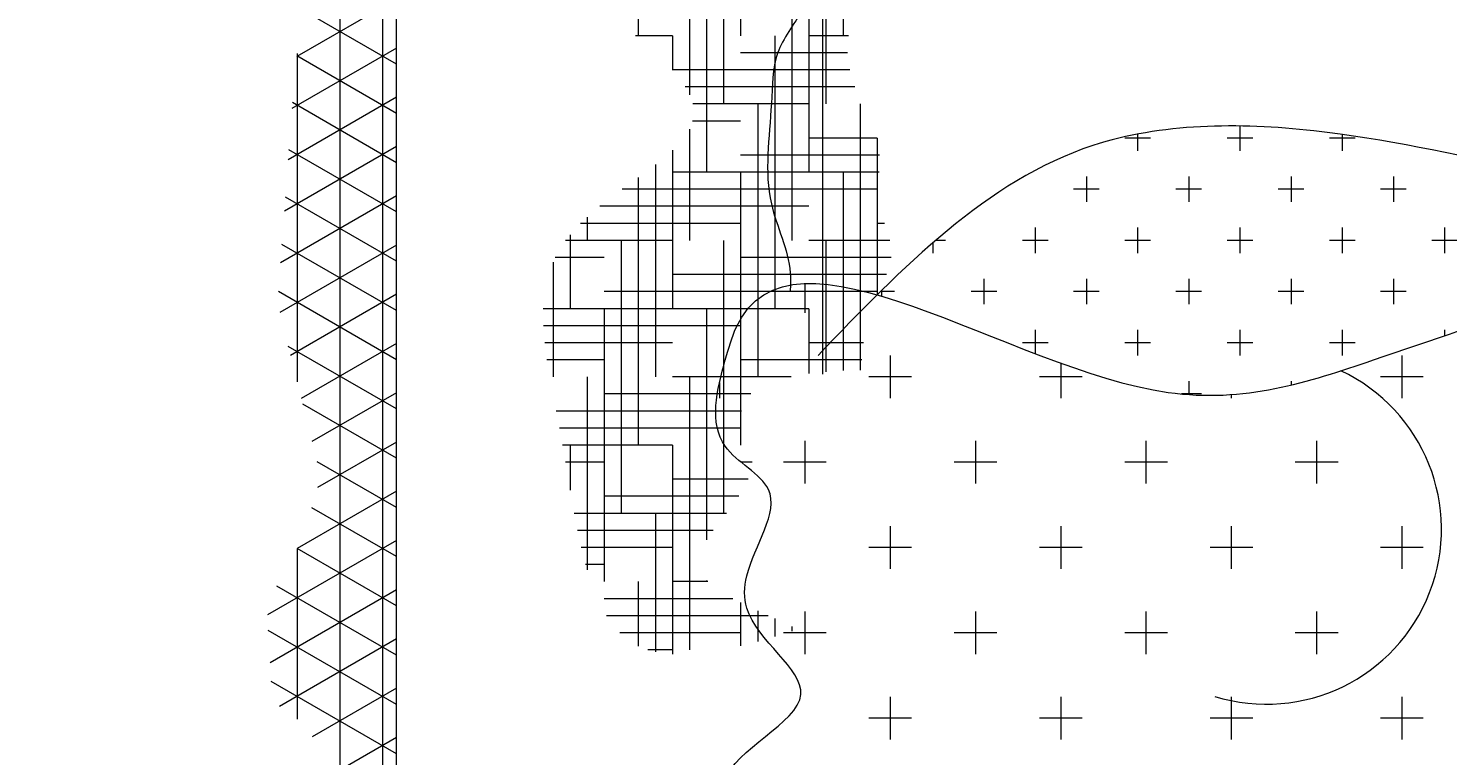
# Model space of a CAD drawing. Units: inches. Extents: x 3731 to 4318, y 1310 to 2388.
# Tile 43 of 57: x 4124 to 4167, y 1977 to 1999. Entities that reach past the tile are written whole.
import ezdxf

# ---------------------------------------------------------------- set-up
doc = ezdxf.new("R2010")
doc.units = ezdxf.units.IN
doc.layers.add('A-ANNO-DIMS', color=2, linetype='Continuous', lineweight=18)
doc.layers.add('A-FURN', color=8, linetype='Continuous', lineweight=13)
doc.styles.get("Standard").update_dxf_attribs({"font": 'arial.ttf'})
doc.dimstyles.get("Standard").update_dxf_attribs({"dimtxt": 0.18, "dimasz": 0.18, "dimexe": 0.18, "dimexo": 0.0625, "dimgap": 0.09, "dimtad": 0, "dimtih": 1, "dimtoh": 1, "dimdec": 4, "dimzin": 0, "dimdsep": 46, "dimtxsty": 'Standard', "dimcen": 0.09, "dimadec": 0, "dimazin": 0, "dimtfac": 1, "dimtdec": 4, "dimtofl": 0, "dimtmove": 0, "dimatfit": 3, "dimfxl": 1, "dimtolj": 1, "dimtzin": 0, "dimarcsym": 0})

# ---------------------------------------------------------------- blocks, each defined once
blk = doc.blocks.new('A$C200C7901')
for p, q in [((2.3121, 1.6596), (2.3121, 0.0201)), ((2, 0.2957), (2, 1.2957)), ((2.0224, 0.9977), (2.0224, 1.1977)), ((2.0224, 0.9977), (2.0224, 1.1977))]:
    blk.add_line(p, q)
at = {"linetype": 'ByBlock'}
for p, q in [((2.3224, 0.0468), (2.3224, 1.6627)), ((2.3224, 0.0468), (2.3224, 1.6627)), ((2.3537, 0.0056), (2.3537, 1.634)), ((2.3537, 0.0056), (2.3537, 1.634)), ((2.3121, 1.5619), (2.3654, 1.5926)), ((2.3121, 1.5619), (2.3654, 1.5926)), ((2.3121, 1.5738), (2.404, 1.5208)), ((2.3121, 1.5738), (2.404, 1.5208)), ((1.5754, 1.532), (1.5754, 1.5633)), ((1.5754, 1.532), (1.5754, 1.5633)), ((1.7004, 1.532), (1.7004, 1.5633)), ((1.7004, 1.532), (1.7004, 1.5633)), ((1.8254, 1.532), (1.8254, 1.5633)), ((1.8254, 1.532), (1.8254, 1.5633)), ((1.9504, 1.532), (1.9504, 1.5633)), ((1.9504, 1.532), (1.9504, 1.5633)), ((2.3121, 1.5258), (2.3739, 1.5615)), ((2.3121, 1.5258), (2.3739, 1.5615)), ((1.5597, 1.5477), (1.591, 1.5477)), ((1.5597, 1.5477), (1.591, 1.5477)), ((1.6847, 1.5477), (1.716, 1.5477)), ((1.6847, 1.5477), (1.716, 1.5477)), ((1.8097, 1.5477), (1.841, 1.5477)), ((1.8097, 1.5477), (1.841, 1.5477)), ((1.9347, 1.5477), (1.966, 1.5477)), ((1.9347, 1.5477), (1.966, 1.5477)), ((2.3121, 1.4897), (2.3979, 1.5393)), ((2.3121, 1.4897), (2.3979, 1.5393)), ((2.3849, 1.4236), (2.3849, 1.5486)), ((2.3849, 1.4236), (2.3849, 1.5486)), ((2.3121, 1.5377), (2.406, 1.4835)), ((2.3121, 1.5377), (2.406, 1.4835)), ((1.6379, 1.4695), (1.6379, 1.5008)), ((1.6379, 1.4695), (1.6379, 1.5008)), ((1.7629, 1.4695), (1.7629, 1.5008)), ((1.7629, 1.4695), (1.7629, 1.5008)), ((1.8879, 1.4695), (1.8879, 1.5008)), ((1.8879, 1.4695), (1.8879, 1.5008)), ((2.0129, 1.4695), (2.0129, 1.5008)), ((2.0129, 1.4695), (2.0129, 1.5008)), ((2.0974, 1.2977), (2.0974, 1.4977)), ((2.0974, 1.2977), (2.0974, 1.4977)), ((2.1099, 1.3477), (2.1099, 1.5009)), ((2.1099, 1.3477), (2.1099, 1.5009)), ((2.1099, 1.4977), (2.1279, 1.4977)), ((2.1099, 1.4977), (2.1279, 1.4977)), ((2.1224, 1.3977), (2.1224, 1.4992)), ((2.1224, 1.3977), (2.1224, 1.4992)), ((2.3121, 1.4537), (2.4047, 1.5071)), ((2.3121, 1.4537), (2.4047, 1.5071)), ((2.3121, 1.5016), (2.3997, 1.4511)), ((2.3121, 1.5016), (2.3997, 1.4511)), ((2.0349, 1.4748), (2.0349, 1.4879)), ((2.0349, 1.4748), (2.0349, 1.4879)), ((2.0474, 1.4691), (2.0474, 1.4915)), ((2.0474, 1.4691), (2.0474, 1.4915)), ((2.0599, 1.4631), (2.0599, 1.4948)), ((2.0599, 1.4631), (2.0599, 1.4948)), ((2.1349, 1.4477), (2.1349, 1.4949)), ((2.1349, 1.4477), (2.1349, 1.4949)), ((1.6222, 1.4852), (1.6535, 1.4852)), ((1.6222, 1.4852), (1.6535, 1.4852)), ((1.7472, 1.4852), (1.7785, 1.4852)), ((1.7472, 1.4852), (1.7785, 1.4852)), ((1.8722, 1.4852), (1.9035, 1.4852)), ((1.8722, 1.4852), (1.9035, 1.4852)), ((1.9972, 1.4852), (2.0285, 1.4852)), ((1.9972, 1.4852), (2.0285, 1.4852)), ((2.0224, 1.4805), (2.0224, 1.4839)), ((2.0224, 1.4805), (2.0224, 1.4839)), ((2.0599, 1.4852), (2.1484, 1.4852)), ((2.0599, 1.4852), (2.1484, 1.4852)), ((2.0397, 1.4727), (2.1581, 1.4727)), ((2.0397, 1.4727), (2.1581, 1.4727)), ((2.3121, 1.4176), (2.4067, 1.4721)), ((2.3121, 1.4176), (2.4067, 1.4721)), ((2.0656, 1.4602), (2.1599, 1.4602)), ((2.0656, 1.4602), (2.1599, 1.4602)), ((2.3121, 1.4655), (2.3849, 1.4235)), ((2.3121, 1.4655), (2.3849, 1.4235)), ((2.084, 1.4477), (2.1099, 1.4477)), ((2.084, 1.4477), (2.1099, 1.4477)), ((2.0849, 1.4468), (2.0849, 1.4477)), ((2.0849, 1.4468), (2.0849, 1.4477)), ((2.1599, 1.2477), (2.1599, 1.4477)), ((2.1599, 1.2477), (2.1599, 1.4477)), ((1.5754, 1.407), (1.5754, 1.4383)), ((1.5754, 1.407), (1.5754, 1.4383)), ((1.7004, 1.407), (1.7004, 1.4383)), ((1.7004, 1.407), (1.7004, 1.4383)), ((1.8254, 1.407), (1.8254, 1.4383)), ((1.8254, 1.407), (1.8254, 1.4383)), ((1.9504, 1.407), (1.9504, 1.4383)), ((1.9504, 1.407), (1.9504, 1.4383)), ((2.1599, 1.4352), (2.1735, 1.4352)), ((2.1599, 1.4352), (2.1735, 1.4352)), ((2.1724, 1.2977), (2.1724, 1.439)), ((2.1724, 1.2977), (2.1724, 1.439)), ((2.3121, 1.4294), (2.3741, 1.3937)), ((2.3121, 1.4294), (2.3741, 1.3937)), ((1.5597, 1.4227), (1.591, 1.4227)), ((1.5597, 1.4227), (1.591, 1.4227)), ((1.6847, 1.4227), (1.716, 1.4227)), ((1.6847, 1.4227), (1.716, 1.4227)), ((1.8097, 1.4227), (1.841, 1.4227)), ((1.8097, 1.4227), (1.841, 1.4227)), ((1.9347, 1.4227), (1.966, 1.4227)), ((1.9347, 1.4227), (1.966, 1.4227)), ((2.0849, 1.2477), (2.0849, 1.4171)), ((2.0849, 1.2477), (2.0849, 1.4171)), ((2.1099, 1.4227), (2.1767, 1.4227)), ((2.1099, 1.4227), (2.1767, 1.4227)), ((2.3121, 1.3815), (2.3848, 1.4235)), ((2.3121, 1.3815), (2.3848, 1.4235)), ((2.08, 1.4102), (2.1795, 1.4102)), ((2.08, 1.4102), (2.1795, 1.4102)), ((2.0703, 1.3977), (2.1819, 1.3977)), ((2.0703, 1.3977), (2.1819, 1.3977)), ((2.0724, 1.1977), (2.0724, 1.3977)), ((2.0724, 1.1977), (2.0724, 1.3977)), ((2.1474, 1.1977), (2.1474, 1.3977)), ((2.1474, 1.1977), (2.1474, 1.3977)), ((2.0612, 1.3852), (2.1599, 1.3852)), ((2.0612, 1.3852), (2.1599, 1.3852)), ((2.3121, 1.3934), (2.3703, 1.3598)), ((2.3121, 1.3934), (2.3703, 1.3598)), ((1.6379, 1.3445), (1.6379, 1.3758)), ((1.6379, 1.3445), (1.6379, 1.3758)), ((1.7629, 1.3445), (1.7629, 1.3758)), ((1.7629, 1.3445), (1.7629, 1.3758)), ((1.8879, 1.3445), (1.8879, 1.3758)), ((1.8879, 1.3445), (1.8879, 1.3758)), ((2.0129, 1.3445), (2.0129, 1.3758)), ((2.0129, 1.3445), (2.0129, 1.3758)), ((2.1849, 1.3477), (2.1849, 1.3808)), ((2.1849, 1.3477), (2.1849, 1.3808)), ((2.3121, 1.3454), (2.37, 1.3788)), ((2.3121, 1.3454), (2.37, 1.3788)), ((2.0545, 1.3727), (2.1099, 1.3727)), ((2.0545, 1.3727), (2.1099, 1.3727)), ((1.6222, 1.3602), (1.6535, 1.3602)), ((1.6222, 1.3602), (1.6535, 1.3602)), ((1.7472, 1.3602), (1.7785, 1.3602)), ((1.7472, 1.3602), (1.7785, 1.3602)), ((1.8722, 1.3602), (1.9035, 1.3602)), ((1.8722, 1.3602), (1.9035, 1.3602)), ((1.9972, 1.3602), (2.0285, 1.3602)), ((1.9972, 1.3602), (2.0285, 1.3602)), ((2.0515, 1.3602), (2.0599, 1.3602)), ((2.0515, 1.3602), (2.0599, 1.3602)), ((2.1599, 1.3602), (2.1883, 1.3602)), ((2.1599, 1.3602), (2.1883, 1.3602)), ((2.3121, 1.3573), (2.3808, 1.3176)), ((2.3121, 1.3573), (2.3808, 1.3176)), ((2.0599, 1.1477), (2.0599, 1.3477)), ((2.0599, 1.1477), (2.0599, 1.3477)), ((2.1099, 1.3477), (2.1904, 1.3477)), ((2.1099, 1.3477), (2.1904, 1.3477)), ((2.1349, 1.1515), (2.1349, 1.3477)), ((2.1349, 1.1515), (2.1349, 1.3477)), ((2.3121, 1.3093), (2.374, 1.345)), ((2.3121, 1.3093), (2.374, 1.345)), ((2.0599, 1.3352), (2.1926, 1.3352)), ((2.0599, 1.3352), (2.1926, 1.3352)), ((2.0594, 1.3227), (2.195, 1.3227)), ((2.0594, 1.3227), (2.195, 1.3227)), ((2.3121, 1.3212), (2.3914, 1.2754)), ((2.3121, 1.3212), (2.3914, 1.2754)), ((1.5754, 1.282), (1.5754, 1.3133)), ((1.5754, 1.282), (1.5754, 1.3133)), ((1.7004, 1.3106), (1.7004, 1.3133)), ((1.7004, 1.3106), (1.7004, 1.3133)), ((1.7316, 1.3008), (1.7316, 1.3106)), ((1.7316, 1.3008), (1.7316, 1.3106)), ((1.8254, 1.2876), (1.8254, 1.3133)), ((1.8254, 1.2876), (1.8254, 1.3133)), ((1.9504, 1.282), (1.9504, 1.3133)), ((1.9504, 1.282), (1.9504, 1.3133)), ((2.0754, 1.3017), (2.0754, 1.3133)), ((2.0754, 1.3017), (2.0754, 1.3133)), ((2.3121, 1.2732), (2.3819, 1.3135)), ((2.3121, 1.2732), (2.3819, 1.3135)), ((1.6566, 1.3008), (1.6566, 1.3036)), ((1.6566, 1.3008), (1.6566, 1.3036)), ((1.7222, 1.3102), (1.7369, 1.3102)), ((1.7222, 1.3102), (1.7369, 1.3102)), ((2.0524, 1.3102), (2.1599, 1.3102)), ((2.0524, 1.3102), (2.1599, 1.3102)), ((2.3849, 1.0607), (2.3849, 1.3013)), ((2.3849, 1.0607), (2.3849, 1.3013)), ((1.5597, 1.2977), (1.591, 1.2977)), ((1.5597, 1.2977), (1.591, 1.2977)), ((1.8097, 1.2977), (1.841, 1.2977)), ((1.8097, 1.2977), (1.841, 1.2977)), ((1.9347, 1.2977), (1.966, 1.2977)), ((1.9347, 1.2977), (1.966, 1.2977)), ((1.9724, 1.0977), (1.9724, 1.2927)), ((1.9724, 1.0977), (1.9724, 1.2927)), ((1.9849, 1.1477), (1.9849, 1.293)), ((1.9849, 1.1477), (1.9849, 1.293)), ((1.9974, 1.1977), (1.9974, 1.2939)), ((1.9974, 1.1977), (1.9974, 1.2939)), ((2.0099, 1.2477), (2.0099, 1.2953)), ((2.0099, 1.2477), (2.0099, 1.2953)), ((2.023, 1.2977), (2.1099, 1.2977)), ((2.023, 1.2977), (2.1099, 1.2977)), ((2.0474, 1.0977), (2.0474, 1.2977)), ((2.0474, 1.0977), (2.0474, 1.2977)), ((2.0597, 1.2977), (2.0744, 1.2977)), ((2.0597, 1.2977), (2.0744, 1.2977)), ((2.1224, 1.1421), (2.1224, 1.2977)), ((2.1224, 1.1421), (2.1224, 1.2977)), ((2.1974, 1.2135), (2.1974, 1.2977)), ((2.1974, 1.2135), (2.1974, 1.2977)), ((1.6191, 1.2633), (1.6191, 1.282)), ((1.6191, 1.2633), (1.6191, 1.282)), ((1.6941, 1.2633), (1.6941, 1.282)), ((1.6941, 1.2633), (1.6941, 1.282)), ((1.7691, 1.2633), (1.7691, 1.282)), ((1.7691, 1.2633), (1.7691, 1.282)), ((1.8441, 1.2633), (1.8441, 1.2806)), ((1.8441, 1.2633), (1.8441, 1.2806)), ((1.9711, 1.2852), (2.0599, 1.2852)), ((1.9711, 1.2852), (2.0599, 1.2852)), ((2.1599, 1.2852), (2.2018, 1.2852)), ((2.1599, 1.2852), (2.2018, 1.2852)), ((2.3121, 1.2851), (2.3985, 1.2352)), ((2.3121, 1.2851), (2.3985, 1.2352)), ((2.3121, 1.2371), (2.3898, 1.282)), ((2.3121, 1.2371), (2.3898, 1.282)), ((1.6097, 1.2727), (1.6285, 1.2727)), ((1.6097, 1.2727), (1.6285, 1.2727)), ((1.6847, 1.2727), (1.7035, 1.2727)), ((1.6847, 1.2727), (1.7035, 1.2727)), ((1.7597, 1.2727), (1.7785, 1.2727)), ((1.7597, 1.2727), (1.7785, 1.2727)), ((1.8347, 1.2727), (1.8535, 1.2727)), ((1.8347, 1.2727), (1.8535, 1.2727)), ((1.97, 1.2727), (2.0099, 1.2727)), ((1.97, 1.2727), (2.0099, 1.2727)), ((2.1099, 1.2727), (2.2034, 1.2727)), ((2.1099, 1.2727), (2.2034, 1.2727)), ((1.5441, 1.2633), (1.5441, 1.2675)), ((1.5441, 1.2633), (1.5441, 1.2675)), ((2.0599, 1.2602), (2.2044, 1.2602)), ((2.0599, 1.2602), (2.2044, 1.2602)), ((2.0129, 1.2293), (2.0129, 1.2508)), ((2.0129, 1.2293), (2.0129, 1.2508)), ((2.3121, 1.2011), (2.3976, 1.2504)), ((2.3121, 1.2011), (2.3976, 1.2504)), ((2.3121, 1.249), (2.396, 1.2006)), ((2.3121, 1.249), (2.396, 1.2006)), ((1.5816, 1.2258), (1.5816, 1.2445)), ((1.5816, 1.2258), (1.5816, 1.2445)), ((1.6566, 1.2258), (1.6566, 1.2445)), ((1.6566, 1.2258), (1.6566, 1.2445)), ((1.7316, 1.2258), (1.7316, 1.2445)), ((1.7316, 1.2258), (1.7316, 1.2445)), ((1.8066, 1.2258), (1.8066, 1.2445)), ((1.8066, 1.2258), (1.8066, 1.2445)), ((1.8816, 1.2258), (1.8816, 1.2445)), ((1.8816, 1.2258), (1.8816, 1.2445)), ((1.9566, 1.2344), (1.9566, 1.2385)), ((1.9566, 1.2344), (1.9566, 1.2385)), ((2.0099, 1.2477), (2.2045, 1.2477)), ((2.0099, 1.2477), (2.2045, 1.2477)), ((2.0349, 1.0477), (2.0349, 1.2477)), ((2.0349, 1.0477), (2.0349, 1.2477)), ((2.1099, 1.1315), (2.1099, 1.2477)), ((2.1099, 1.1315), (2.1099, 1.2477)), ((2.1849, 1.1935), (2.1849, 1.2477)), ((2.1849, 1.1935), (2.1849, 1.2477)), ((1.5722, 1.2352), (1.591, 1.2352)), ((1.5722, 1.2352), (1.591, 1.2352)), ((1.6472, 1.2352), (1.666, 1.2352)), ((1.6472, 1.2352), (1.666, 1.2352)), ((1.7222, 1.2352), (1.741, 1.2352)), ((1.7222, 1.2352), (1.741, 1.2352)), ((1.7972, 1.2352), (1.816, 1.2352)), ((1.7972, 1.2352), (1.816, 1.2352)), ((1.8722, 1.2352), (1.891, 1.2352)), ((1.8722, 1.2352), (1.891, 1.2352)), ((1.9472, 1.2352), (1.9574, 1.2352)), ((1.9472, 1.2352), (1.9574, 1.2352)), ((1.9599, 1.1228), (1.9599, 1.2373)), ((1.9599, 1.1228), (1.9599, 1.2373)), ((1.9599, 1.2352), (2.1599, 1.2352)), ((1.9599, 1.2352), (2.1599, 1.2352)), ((2, 1.2352), (2.0285, 1.2352)), ((2, 1.2352), (2.0285, 1.2352)), ((1.953, 1.2227), (2.1099, 1.2227)), ((1.953, 1.2227), (2.1099, 1.2227)), ((1.5441, 1.1883), (1.5441, 1.207)), ((1.5441, 1.1883), (1.5441, 1.207)), ((1.6191, 1.1883), (1.6191, 1.207)), ((1.6191, 1.1883), (1.6191, 1.207)), ((1.6941, 1.1883), (1.6941, 1.207)), ((1.6941, 1.1883), (1.6941, 1.207)), ((1.7691, 1.1883), (1.7691, 1.207)), ((1.7691, 1.1883), (1.7691, 1.207)), ((1.8441, 1.1883), (1.8441, 1.207)), ((1.8441, 1.1883), (1.8441, 1.207)), ((1.9191, 1.1995), (1.9191, 1.207)), ((1.9191, 1.1995), (1.9191, 1.207)), ((1.9495, 1.2102), (2.0599, 1.2102)), ((1.9495, 1.2102), (2.0599, 1.2102)), ((2.1599, 1.2102), (2.1959, 1.2102)), ((2.1599, 1.2102), (2.1959, 1.2102)), ((2.3121, 1.165), (2.397, 1.214)), ((2.3121, 1.165), (2.397, 1.214)), ((2.3121, 1.2129), (2.3935, 1.166)), ((2.3121, 1.2129), (2.3935, 1.166)), ((1.5347, 1.1977), (1.5535, 1.1977)), ((1.5347, 1.1977), (1.5535, 1.1977)), ((1.6097, 1.1977), (1.6285, 1.1977)), ((1.6097, 1.1977), (1.6285, 1.1977)), ((1.6847, 1.1977), (1.7035, 1.1977)), ((1.6847, 1.1977), (1.7035, 1.1977)), ((1.7597, 1.1977), (1.7785, 1.1977)), ((1.7597, 1.1977), (1.7785, 1.1977)), ((1.8347, 1.1977), (1.8535, 1.1977)), ((1.8347, 1.1977), (1.8535, 1.1977)), ((1.9097, 1.1977), (1.917, 1.1977)), ((1.9097, 1.1977), (1.917, 1.1977)), ((1.9506, 1.1977), (2.0099, 1.1977)), ((1.9506, 1.1977), (2.0099, 1.1977)), ((2.0974, 1.1161), (2.0974, 1.1977)), ((2.0974, 1.1161), (2.0974, 1.1977)), ((2.1099, 1.1977), (2.1882, 1.1977)), ((2.1099, 1.1977), (2.1882, 1.1977)), ((2.1724, 1.1807), (2.1724, 1.1977)), ((2.1724, 1.1807), (2.1724, 1.1977)), ((1.9545, 1.1852), (1.9599, 1.1852)), ((1.9545, 1.1852), (1.9599, 1.1852)), ((2.0599, 1.1852), (2.1772, 1.1852)), ((2.0599, 1.1852), (2.1772, 1.1852)), ((2.3121, 1.1768), (2.3909, 1.1314)), ((2.3121, 1.1768), (2.3909, 1.1314)), ((2.3121, 1.1289), (2.3942, 1.1763)), ((2.3121, 1.1289), (2.3942, 1.1763)), ((1.5816, 1.1508), (1.5816, 1.1695)), ((1.5816, 1.1508), (1.5816, 1.1695)), ((1.6566, 1.1508), (1.6566, 1.1695)), ((1.6566, 1.1508), (1.6566, 1.1695)), ((1.7316, 1.1508), (1.7316, 1.1695)), ((1.7316, 1.1508), (1.7316, 1.1695)), ((1.8066, 1.1508), (1.8066, 1.1695)), ((1.8066, 1.1508), (1.8066, 1.1695)), ((2.0099, 1.1727), (2.1631, 1.1727)), ((2.0099, 1.1727), (2.1631, 1.1727)), ((1.5722, 1.1602), (1.591, 1.1602)), ((1.5722, 1.1602), (1.591, 1.1602)), ((1.6472, 1.1602), (1.666, 1.1602)), ((1.6472, 1.1602), (1.666, 1.1602)), ((1.7222, 1.1602), (1.741, 1.1602)), ((1.7222, 1.1602), (1.741, 1.1602)), ((1.7972, 1.1602), (1.816, 1.1602)), ((1.7972, 1.1602), (1.816, 1.1602)), ((1.9599, 1.1602), (2.1468, 1.1602)), ((1.9599, 1.1602), (2.1468, 1.1602)), ((1.9585, 1.1477), (2.1099, 1.1477)), ((1.9585, 1.1477), (2.1099, 1.1477)), ((2.0099, 0.9477), (2.0099, 1.1477)), ((2.0099, 0.9477), (2.0099, 1.1477)), ((2.0849, 0.9477), (2.0849, 1.1477)), ((2.0849, 0.9477), (2.0849, 1.1477)), ((1.9581, 1.1352), (2.0599, 1.1352)), ((1.9581, 1.1352), (2.0599, 1.1352)), ((2.3121, 1.1408), (2.3884, 1.0967)), ((2.3121, 1.1408), (2.3884, 1.0967)), ((2.3121, 1.0928), (2.3915, 1.1386)), ((2.3121, 1.0928), (2.3915, 1.1386)), ((1.6191, 1.1201), (1.6191, 1.132)), ((1.6191, 1.1201), (1.6191, 1.132)), ((1.6941, 1.1139), (1.6941, 1.132)), ((1.6941, 1.1139), (1.6941, 1.132)), ((1.7691, 1.1198), (1.7691, 1.132)), ((1.7691, 1.1198), (1.7691, 1.132)), ((1.6097, 1.1227), (1.6285, 1.1227)), ((1.6097, 1.1227), (1.6285, 1.1227)), ((1.6847, 1.1227), (1.7035, 1.1227)), ((1.6847, 1.1227), (1.7035, 1.1227)), ((1.7597, 1.1227), (1.7785, 1.1227)), ((1.7597, 1.1227), (1.7785, 1.1227)), ((1.9599, 1.1227), (2.0099, 1.1227)), ((1.9599, 1.1227), (2.0099, 1.1227)), ((2.0599, 1.1102), (2.0951, 1.1102)), ((2.0599, 1.1102), (2.0951, 1.1102)), ((2.3121, 1.1047), (2.3851, 1.0625)), ((2.3121, 1.1047), (2.3851, 1.0625)), ((1.9974, 0.8977), (1.9974, 1.0977)), ((1.9974, 0.8977), (1.9974, 1.0977)), ((2.0099, 1.0977), (2.095, 1.0977)), ((2.0099, 1.0977), (2.095, 1.0977)), ((2.0724, 0.8977), (2.0724, 1.0977)), ((2.0724, 0.8977), (2.0724, 1.0977)), ((2.3121, 1.0567), (2.3887, 1.1009)), ((2.3121, 1.0567), (2.3887, 1.1009)), ((1.9763, 1.0852), (2.1005, 1.0852)), ((1.9763, 1.0852), (2.1005, 1.0852)), ((2.0974, 0.9977), (2.0974, 1.0909)), ((2.0974, 0.9977), (2.0974, 1.0909)), ((1.9799, 1.0727), (2.1099, 1.0727)), ((1.9799, 1.0727), (2.1099, 1.0727)), ((2.1099, 1.0477), (2.1099, 1.0729)), ((2.1099, 1.0477), (2.1099, 1.0729)), ((2.3121, 1.0686), (2.3813, 1.0286)), ((2.3121, 1.0686), (2.3813, 1.0286)), ((2.3121, 1.0206), (2.3851, 1.0628)), ((2.3121, 1.0206), (2.3851, 1.0628)), ((1.9815, 1.0602), (2.0599, 1.0602)), ((1.9815, 1.0602), (2.0599, 1.0602)), ((1.981, 1.0477), (2.0099, 1.0477)), ((1.981, 1.0477), (2.0099, 1.0477)), ((1.9849, 0.9171), (1.9849, 1.0477)), ((1.9849, 0.9171), (1.9849, 1.0477)), ((2.0599, 0.8477), (2.0599, 1.0477)), ((2.0599, 0.8477), (2.0599, 1.0477)), ((2.1099, 1.0477), (2.137, 1.0477)), ((2.1099, 1.0477), (2.137, 1.0477)), ((2.1349, 0.8477), (2.1349, 1.0477)), ((2.1349, 0.8477), (2.1349, 1.0477))]:
    blk.add_line(p, q, dxfattribs=at)
blk.add_arc((1.6746, 1.4093), 0.1282, 72.7909, 244.8695, dxfattribs=at)
blk.add_arc((1.6746, 1.4093), 0.1282, 72.7909, 244.8695, dxfattribs=at)
for points, knots in [([(0.4485, 1.7835), (0.4321, 1.7496), (0.4062, 1.6964), (0.49, 1.6713), (0.4719, 1.5969), (0.4123, 1.592), (0.4233, 1.5337), (0.4954, 1.5086), (0.4012, 1.4738), (0.3253, 1.4306), (0.4113, 1.3764), (0.3688, 1.3065), (0.5579, 1.2663), (0.741, 1.4533), (1.1127, 1.1109), (1.4811, 1.2478), (1.7885, 1.3492), (2.0357, 1.1637), (2.0748, 1.2974), (2.0876, 1.349), (2.0192, 1.3805), (2.0564, 1.4298), (2.0588, 1.4846), (1.9759, 1.5349), (2.1004, 1.5845), (2.0397, 1.6519), (1.971, 1.7053), (2.1104, 1.8981), (1.5946, 1.7967), (1.2448, 1.7472), (0.8129, 1.7935), (0.4953, 1.8548), (0.4582, 1.7983), (0.4485, 1.7835)], [0, 0, 0, 0, 88.420092, 139.08588, 204.302936, 239.695496, 287.801042, 327.365471, 412.960499, 463.626286, 552.059846, 584.668336, 662.614915, 940.993281, 1309.926334, 1844.022653, 1996.276242, 2316.43048, 2341.441004, 2404.707416, 2449.463774, 2514.680778, 2538.40571, 2613.031547, 2697.13096, 2760.903931, 2822.692699, 2945.47, 3215.060018, 3725.584917, 4361.974444, 4504.671998, 4555.32777, 4555.32777, 4555.32777, 4555.32777]), ([(0.4856, 1.3429), (0.5504, 1.3182), (0.6715, 1.2721), (0.8374, 1.0498), (1.1164, 1.1183), (1.3878, 1.1816), (1.5888, 1.1102), (1.8403, 1.1127), (1.9415, 1.2178), (2.0032, 1.2819)], [0, 0, 0, 0, 205.411753, 383.654933, 772.067458, 921.644661, 1226.793228, 1388.983508, 1642.292305, 1642.292305, 1642.292305, 1642.292305])]:
    blk.add_open_spline(points, degree=3, knots=knots)
blk.add_open_spline([(0.473, 1.2954), (0.4739, 1.2781), (0.4755, 1.2477), (0.5032, 1.2084), (0.4801, 1.1701), (0.4928, 1.1255), (0.4674, 1.0912), (0.4579, 1.0351), (0.501, 0.9724), (0.4311, 0.8832), (0.4902, 0.8637), (0.4843, 0.8288), (0.4774, 0.7906), (0.4625, 0.7457), (0.459, 0.6999), (0.4816, 0.6664), (0.4748, 0.625), (0.4791, 0.5889), (0.4533, 0.5528), (0.4738, 0.5004), (0.4658, 0.4502), (0.4696, 0.3946), (0.4189, 0.3935), (0.4493, 0.3684), (0.4694, 0.3857), (0.4922, 0.3576), (0.5297, 0.3262), (0.5917, 0.3353), (0.6454, 0.3754), (0.7083, 0.3741), (0.7643, 0.3328), (0.826, 0.346), (0.925, 0.3388), (1.0353, 0.3593), (1.1561, 0.3744), (1.2477, 0.3154), (1.3302, 0.3474), (1.4086, 0.3512), (1.5217, 0.3878), (1.6362, 0.3176), (1.7682, 0.3285), (1.8402, 0.3019), (1.9071, 0.3529), (1.9647, 0.3412), (2.0795, 0.2948), (2.0472, 0.3498), (2.0343, 0.3772), (2.0435, 0.43), (2.0109, 0.5782), (2.0746, 0.4643), (2.0805, 0.584), (2.0084, 0.5979), (2.0343, 0.6846), (2.0344, 0.746), (2.0293, 0.8096), (2.0489, 0.8545), (2.0652, 0.9218), (1.9842, 0.9297), (2.0007, 1.0162), (2.0367, 1.0585), (2.0367, 1.1102), (2.0457, 1.1647), (2.0226, 1.2084), (2.0234, 1.2306), (2.0236, 1.2352)], degree=3, knots=[0, 0, 0, 0, 51.660678, 90.967412, 128.902454, 170.303599, 219.852997, 247.834962, 336.321557, 429.35469, 458.821847, 477.222321, 524.135809, 581.038434, 617.839381, 657.146115, 693.947125, 740.178081, 760.753248, 820.731705, 885.133458, 928.777044, 953.563729, 976.574207, 995.553042, 1018.563482, 1064.584401, 1147.951297, 1174.787598, 1266.851571, 1308.018447, 1377.066427, 1441.511314, 1608.245014, 1714.11869, 1792.771707, 1913.247991, 1954.931389, 2029.864445, 2259.189419, 2305.221512, 2429.507982, 2456.344283, 2543.92595, 2627.925037, 2662.96218, 2687.736879, 2719.937755, 2839.540991, 2875.47895, 2953.681041, 2993.270313, 3066.872333, 3154.395764, 3200.397042, 3248.426375, 3312.828127, 3347.881398, 3444.484026, 3481.577522, 3518.665244, 3592.267265, 3644.719162, 3658.519501, 3658.519501, 3658.519501, 3658.519501], dxfattribs=at)
blk = doc.blocks.new('*D38')
at = {"layer": 'A-ANNO-DIMS', "color": 0, "lineweight": -2, "transparency": 16777216}
for p, q in [((4103.271, 2262.382), (4318.341, 2262.382)), ((4318.161, 2262.202), (4318.161, 2103.064)), ((4318.161, 1943.562), (4318.161, 2102.7)), ((4234.271, 1943.382), (4318.341, 1943.382))]:
    blk.add_line(p, q, dxfattribs=at)
at = {"layer": 'A-ANNO-DIMS', "color": 0, "transparency": 16777216}
for points in [[(4318.131, 2262.202), (4318.191, 2262.202), (4318.161, 2262.382)], [(4318.131, 1943.562), (4318.191, 1943.562), (4318.161, 1943.382)]]:
    blk.add_solid(points, dxfattribs=at)
at = {"layer": 'Defpoints', "color": 0, "transparency": 16777216}
for p in [(4103.209, 2262.382), (4318.161, 2262.382), (4234.209, 1943.382)]:
    blk.add_point(p, dxfattribs=at)
at = {"layer": 'A-ANNO-DIMS', "color": 0, "transparency": 16777216, "insert": (4318.161, 2102.882), "char_height": 0.18, "attachment_point": 5}
blk.add_mtext('\\A1;319', dxfattribs=at)

msp = doc.modelspace()

# ---------------------------------------------------------------- block references
at = {"layer": 'A-FURN', "xscale": 41.1071563136412, "yscale": 41.1071563136412, "zscale": 41.1071563136412, "rotation": 180}
msp.add_blockref('A$C200C7901', (4230.145, 2042.037), dxfattribs=at)

# ---------------------------------------------------------------- dimensions: what is measured, and where the dimension line sits
at = {"layer": 'A-ANNO-DIMS'}
dim = msp.add_linear_dim(base=(4318.161, 2262.382), p1=(4234.209, 1943.382), p2=(4103.209, 2262.382), angle=90, dimstyle='Standard', override={"dimdec": 0, "dimlfac": 1, "dimrnd": 0, "dimzin": 0, "dimdsep": 46, "dimlunit": 2}, dxfattribs=at)
dim.commit()
dim.dimension.update_dxf_attribs({"geometry": '*D38', "text_midpoint": (4318.161, 2102.882)})

doc.saveas('drawing.dxf')
